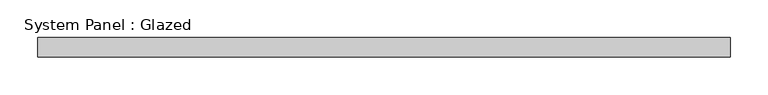
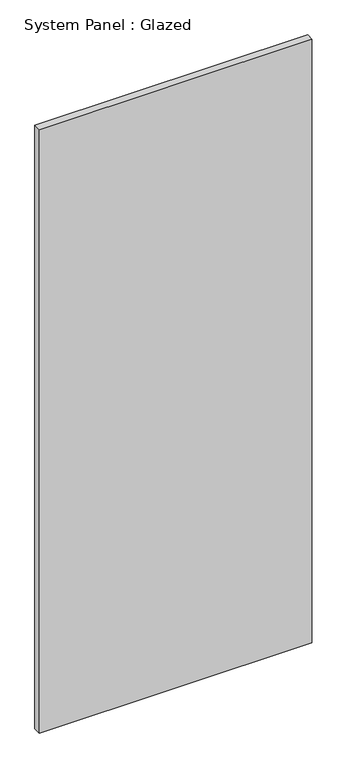
"""IFC4 building model written with IfcOpenShell, lengths in millimetres: plate geometry, System Panel : Glazed."""

from ifc_helpers import new_model, si_unit, origin, origin_with_axes, place, context, project, spatial, polyline, outline, extrude, source, transform, mapped, element, save


def system_panel_glazed_14bb7e7b(model_context):
    return source(origin(), model_context, "Body", "SweptSolid", [
        extrude(outline(polyline([(457.2, 19.05), (-457.2, 19.05), (-457.2, 44.45), (457.2, 44.45), (457.2, 19.05)])), origin_with_axes(), (0.0, 0.0, 1.0), 2139.95),
    ])


if __name__ == "__main__":
    model = new_model("IFC4")
    model_context = context("Model", 3, world=origin())
    ifc_project = project(units=[si_unit("LENGTHUNIT", "METRE", prefix="MILLI")], contexts=[model_context])
    site = spatial("IfcSite", under=ifc_project)
    building = spatial("IfcBuilding", under=site)
    placement = place(None, origin())
    system_panel_glazed_shape = system_panel_glazed_14bb7e7b(model_context)
    element("IfcPlate", 1, ObjectType="System Panel : Glazed", at=placement, inside=building, context=model_context, shape_type="MappedRepresentation", body=[
        mapped(system_panel_glazed_shape, transform((0.0, 0.0, 0.0), x_axis=(1.0, 0.0, 0.0), y_axis=(0.0, 1.0, 0.0), z_axis=(0.0, 0.0, 1.0))),
    ])
    save(model, "model.ifc")

# Revit data of these elements
# Type "System Panel : Glazed"
#   Construction Type Id = "GSP4R"
#   Analytic Construction = "1/8 in Pilkington single glazing"
#   Visual Light Transmittance = 0.9
#   Solar Heat Gain Coefficient = 0.86
#   Heat Transfer Coefficient (U) = 1.18115 BTU/(h·ft²·°F)
# Element 1 (IfcPlate, "System Panel : Glazed")
#   Materials on its faces: "Glass"
# Materials
#   "Glass": class "Glass", colour RGB 0 128 192, transparency 0.75, Description = "Soda Lime Glass", Cost = 0
